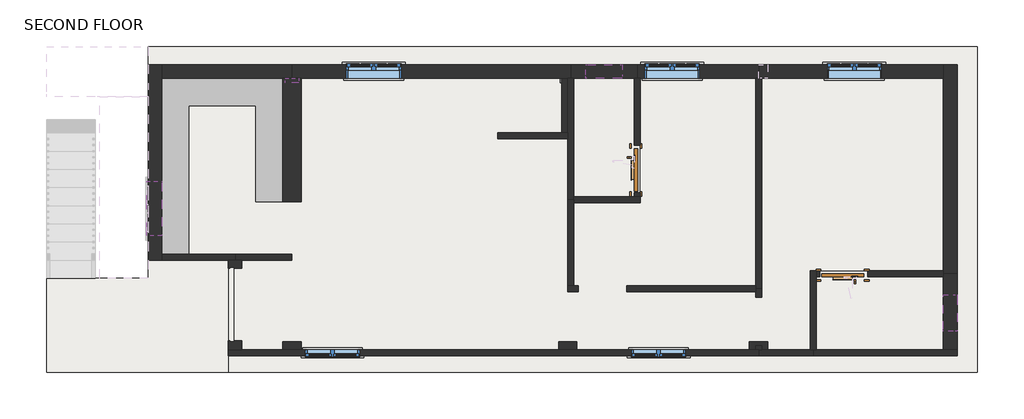
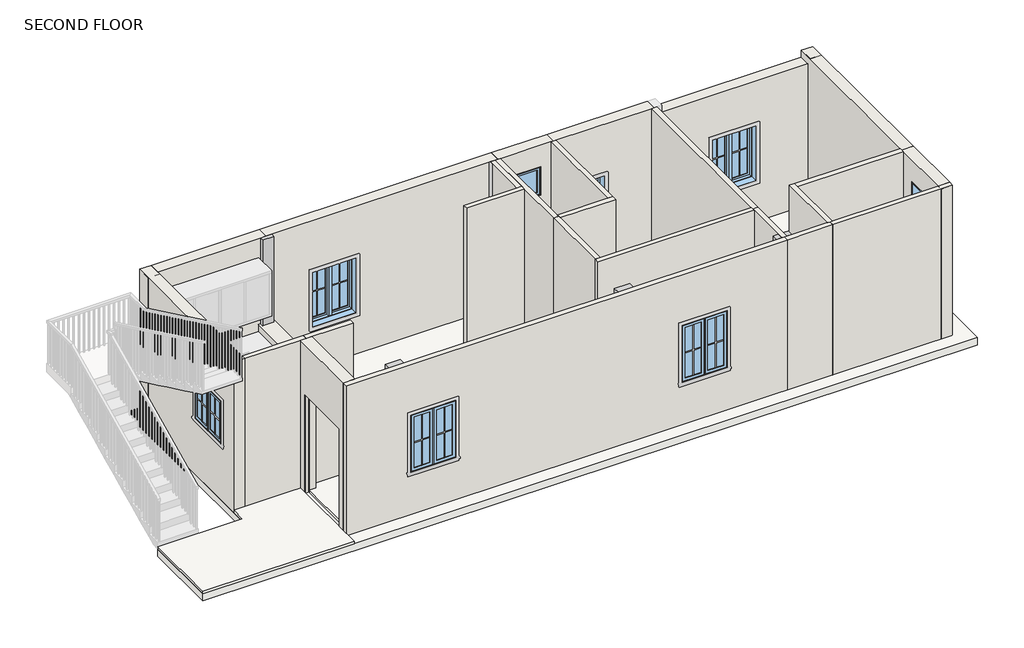
# One storey, part 1 of 3: 26 walls, 8 windows, 6 columns, 4 slabs, 2 doors.
"""IFC4 building model written with IfcOpenShell, lengths in millimetres."""

from ifc_helpers import new_model, si_unit, frame, origin, place, context, project, spatial, polyline, outline, extrude, faceted_brep, transform, mapped, element, save
from components import apartment_toilet_door_15897_d3_toilet_d7560075, apartment_toilet_door_15897_d3_toilet_03746f18, window_80340324, window_casement_double_w1_d341e8ac, window_casement_double_w1_80f1179f, window_casement_double_w1_2_90de19e9

model = new_model("IFC4")

# Units and contexts
model_context = context("Model", 3, world=origin())
ifc_project = project(units=[si_unit("LENGTHUNIT", "METRE", prefix="MILLI")], contexts=[model_context])

# Site, building, storey
site = spatial("IfcSite", under=ifc_project)
building = spatial("IfcBuilding", under=site)
storey = spatial("IfcBuildingStorey", under=building, Name="SECOND FLOOR", Elevation=6400.8)

# Columns
placement = place(None, origin())
element("IfcColumn", 1, ObjectType="Rectangular Column : 9\" X 12\"", at=placement, inside=storey, context=model_context, shape_type="SweptSolid", body=[
    extrude(outline(polyline([(-2166.0591227, 4797.7642852), (-2394.6591227, 4797.7642852), (-2394.6591227, 4873.9642852), (-2280.3591227, 4873.9642852), (-2166.0591227, 4873.9642852), (-2166.0591227, 4797.7642852)])), frame((0.0, 0.0, 7772.4), z_axis=(0.0, 0.0, 1.0), x_axis=(1.0, 0.0, 0.0)), (0.0, 0.0, 1.0), 1828.8),
])
element("IfcColumn", 2, ObjectType="Rectangular Column : 9\" X 12\"", at=placement, inside=storey, context=model_context, shape_type="Brep", body=[
    faceted_brep([(-4693.3591227, 5102.5642852, 6400.8), (-4464.7591227, 5102.5642852, 6400.8), (-4464.7591227, 4873.9642852, 6400.8), (-4464.7591227, 4797.7642852, 6400.8), (-4693.3591227, 4797.7642852, 6400.8), (-4693.3591227, 5102.5642852, 9601.2), (-4464.7591227, 5102.5642852, 9601.2), (-4464.7591227, 4873.9642852, 9601.2), (-4464.7591227, 4797.7642852, 9601.2), (-4693.3591227, 4797.7642852, 9601.2)], [[[0, 1, 2, 3, 4]], [[5, 6, 1, 0]], [[6, 7, 8, 3, 2, 1]], [[8, 9, 4, 3]], [[9, 5, 0, 4]], [[5, 9, 8, 7, 6]]]),
])
element("IfcColumn", 3, ObjectType="Rectangular Column : 9\" X 12\"", at=placement, inside=storey, context=model_context, shape_type="Brep", body=[
    faceted_brep([(5390.4408773, 454.3642852, 6400.8), (5695.2408773, 454.3642852, 6400.8), (5695.2408773, 327.3642852, 6400.8), (5593.6408773, 327.3642852, 6400.8), (5593.6408773, 390.8642852, 6400.8), (5492.0408773, 390.8642852, 6400.8), (5492.0408773, 327.3642852, 6400.8), (5390.4408773, 327.3642852, 6400.8), (5695.2408773, 454.3642852, 9601.2), (5695.2408773, 327.3642852, 9601.2), (5390.4408773, 454.3642852, 9601.2), (5390.4408773, 327.3642852, 9601.2), (5492.0408773, 454.3642852, 9601.2), (5492.0408773, 454.3642852, 8534.4), (5593.6408773, 454.3642852, 8534.4), (5593.6408773, 454.3642852, 9601.2), (5593.6408773, 327.3642852, 9601.2), (5593.6408773, 390.8642852, 8534.4), (5492.0408773, 390.8642852, 8534.4), (5492.0408773, 327.3642852, 9601.2)], [[[0, 1, 2, 3, 4, 5, 6, 7]], [[1, 8, 9, 2]], [[10, 0, 7, 11]], [[1, 0, 10, 12, 13, 14, 15, 8]], [[8, 15, 16, 9]], [[17, 4, 3, 16, 15, 14]], [[5, 18, 13, 12, 19, 6]], [[4, 17, 18, 5]], [[18, 17, 14, 13]], [[7, 6, 19, 11]], [[12, 10, 11, 19]], [[3, 2, 9, 16]]]),
])
element("IfcColumn", 4, ObjectType="Rectangular Column : 9\" X 12\"", at=placement, inside=storey, context=model_context, shape_type="SweptSolid", body=[
    extrude(outline(polyline([(2190.0408773, 454.3642852), (2494.8408773, 454.3642852), (2494.8408773, 327.3642852), (2190.0408773, 327.3642852), (2190.0408773, 454.3642852)])), frame((0.0, 0.0, 6400.8), z_axis=(0.0, 0.0, 1.0), x_axis=(1.0, 0.0, 0.0)), (0.0, 0.0, 1.0), 3200.4),
])
element("IfcColumn", 5, ObjectType="Rectangular Column : 9\" X 12\"", at=placement, inside=storey, context=model_context, shape_type="SweptSolid", body=[
    extrude(outline(polyline([(-2432.7591227, 454.3642852), (-2127.9591227, 454.3642852), (-2127.9591227, 327.3642852), (-2432.7591227, 327.3642852), (-2432.7591227, 454.3642852)])), frame((0.0, 0.0, 6400.8), z_axis=(0.0, 0.0, 1.0), x_axis=(1.0, 0.0, 0.0)), (0.0, 0.0, 1.0), 3200.4),
])
element("IfcColumn", 6, ObjectType="Rectangular Column : 9\" X 12\"", at=placement, inside=storey, context=model_context, shape_type="Brep", body=[
    faceted_brep([(-4693.3591227, 2130.7642852, 6400.8), (-4464.7591227, 2130.7642852, 6400.8), (-4464.7591227, 1927.5642852, 6400.8), (-4464.7591227, 1825.9642852, 6400.8), (-4693.3591227, 1825.9642852, 6400.8), (-4693.3591227, 2130.7642852, 9601.2), (-4464.7591227, 2130.7642852, 9601.2), (-4464.7591227, 1927.5642852, 9601.2), (-4464.7591227, 1825.9642852, 9601.2), (-4693.3591227, 1825.9642852, 9601.2)], [[[0, 1, 2, 3, 4]], [[5, 6, 1, 0]], [[6, 7, 8, 3, 2, 1]], [[8, 9, 4, 3]], [[9, 5, 0, 4]], [[5, 9, 8, 7, 6]]]),
])

# Doors
apartment_toilet_door_15897_d3_toilet_shape = apartment_toilet_door_15897_d3_toilet_d7560075(model_context)
element("IfcDoor", 7, ObjectType="Apartment_Toilet_Door_15897 : D3 TOILET", at=placement, inside=storey, context=model_context, shape_type="MappedRepresentation", body=[
    mapped(apartment_toilet_door_15897_d3_toilet_shape, transform((6952.5408773, 1597.3642852, 6400.8), x_axis=(-1.0, 0.0, 0.0), y_axis=(0.0, -1.0, 0.0), z_axis=(0.0, 0.0, 1.0))),
])
apartment_toilet_door_15897_d3_toilet_2_shape = apartment_toilet_door_15897_d3_toilet_03746f18(model_context)
element("IfcDoor", 8, ObjectType="Apartment_Toilet_Door_15897 : D3 TOILET", at=placement, inside=storey, context=model_context, shape_type="MappedRepresentation", body=[
    mapped(apartment_toilet_door_15897_d3_toilet_2_shape, transform((3510.8408773, 3337.2642852, 6400.8), x_axis=(0.0, -1.0, 0.0), y_axis=(1.0, 0.0, 0.0), z_axis=(0.0, 0.0, 1.0))),
])

# Slabs
element("IfcSlab", 9, ObjectType="6\" SLAB", at=placement, inside=storey, context=model_context, shape_type="SweptSolid", body=[
    extrude(outline(polyline([(9213.1408773, 5407.3642852), (9213.1408773, 113.4304234), (9213.1408773, -53.6357148), (-6395.1591227, -53.6357148), (-6395.1591227, 1521.1642852), (-4693.3591227, 1521.1642852), (-4693.3591227, 5407.3642852), (9213.1408773, 5407.3642852)])), frame((0.0, 0.0, 6248.4), z_axis=(0.0, 0.0, 1.0), x_axis=(1.0, 0.0, 0.0)), (0.0, 0.0, 1.0), 152.4),
])
element("IfcSlab", 10, ObjectType="FLOORING", at=placement, inside=storey, context=model_context, shape_type="SweptSolid", body=[
    extrude(outline(polyline([(-4464.7591227, 1927.5642852), (-4464.7591227, 4873.9642852), (-2432.7591227, 4873.9642852), (-2432.7591227, 2803.8642852), (-2127.9591227, 2803.8642852), (-2127.9591227, 4873.9642852), (2240.8408773, 4873.9642852), (2240.8408773, 3959.5642852), (1174.0408773, 3959.5642852), (1174.0408773, 3857.9642852), (2342.4408773, 3857.9642852), (2342.4408773, 1292.5642852), (2520.2408773, 1292.5642852), (2520.2408773, 1394.1642852), (2444.0408773, 1394.1642852), (2444.0408773, 2791.1642852), (3561.6408773, 2791.1642852), (3561.6408773, 4873.9642852), (5492.0408773, 4873.9642852), (5492.0408773, 1394.1642852), (3409.2408773, 1394.1642852), (3333.0408773, 1394.1642852), (3333.0408773, 1292.5642852), (5492.0408773, 1292.5642852), (5492.0408773, 1203.6642852), (5593.6408773, 1203.6642852), (5593.6408773, 4873.9642852), (8641.6408773, 4873.9642852), (8641.6408773, 1648.1642852), (6406.4408773, 1648.1642852), (6406.4408773, 327.3642852), (5593.6408773, 327.3642852), (5593.6408773, 390.8642852), (5492.0408773, 390.8642852), (5492.0408773, 327.3642852), (-3118.5591227, 327.3642852), (-3118.5591227, 397.6642852), (-3250.1591227, 397.6642852), (-3250.1591227, 1769.2642852), (-3118.5591227, 1769.2642852), (-3118.5591227, 1825.9642852), (-2280.3591227, 1825.9642852), (-2280.3591227, 1927.5642852), (-4464.7591227, 1927.5642852)])), frame((0.0, 0.0, 6400.8), z_axis=(0.0, 0.0, 1.0), x_axis=(1.0, 0.0, 0.0)), (0.0, 0.0, 1.0), 50.8),
])
element("IfcSlab", 11, ObjectType="FLOORING OPEN AREA", at=placement, inside=storey, context=model_context, shape_type="SweptSolid", body=[
    extrude(outline(polyline([(-3347.1591227, -53.6357148), (-6395.1591227, -53.6357148), (-6395.1591227, 1521.1642852), (-4693.3591227, 1521.1642852), (-4693.3591227, 1825.9642852), (-3347.1591227, 1825.9642852), (-3347.1591227, -53.6357148)])), frame((0.0, 0.0, 6400.8), z_axis=(0.0, 0.0, 1.0), x_axis=(1.0, 0.0, 0.0)), (0.0, 0.0, 1.0), 50.8),
])
element("IfcSlab", 12, ObjectType="FLOORING TOILET", at=placement, inside=storey, context=model_context, shape_type="SweptSolid", body=[
    extrude(outline(polyline([(7371.5408773, 1546.5642852), (8641.6408773, 1546.5642852), (8641.6408773, 327.3642852), (6508.0408773, 327.3642852), (6508.0408773, 1546.5642852), (6571.5408773, 1546.5642852), (6571.5408773, 1648.1642852), (7371.5408773, 1648.1642852), (7371.5408773, 1546.5642852)])), frame((0.0, 0.0, 6400.8), z_axis=(0.0, 0.0, 1.0), x_axis=(1.0, 0.0, 0.0)), (0.0, 0.0, 1.0), 50.8),
    extrude(outline(polyline([(3460.0408773, 4873.9642852), (3460.0408773, 3756.2642852), (3561.6408773, 3756.2642852), (3561.6408773, 2956.2642852), (3460.0408773, 2956.2642852), (3460.0408773, 2892.7642852), (2444.0408773, 2892.7642852), (2444.0408773, 4873.9642852), (3460.0408773, 4873.9642852)])), frame((0.0, 0.0, 6400.8), z_axis=(0.0, 0.0, 1.0), x_axis=(1.0, 0.0, 0.0)), (0.0, 0.0, 1.0), 50.8),
])

# Walls
element("IfcWall", 13, at=placement, inside=storey, context=model_context, shape_type="Brep", body=[
    faceted_brep([(-2432.7591227, 4873.9642852, 6400.8), (-2432.7591227, 2803.8642852, 6400.8), (-2432.7591227, 2803.8642852, 7772.4), (-2432.7591227, 4873.9642852, 7772.4), (-2127.9591227, 4873.9642852, 6400.8), (-2127.9591227, 4873.9642852, 7772.4), (-2127.9591227, 2803.8642852, 7772.4), (-2127.9591227, 2803.8642852, 6400.8), (-2280.3591227, 4873.9642852, 6400.8), (-2166.0591227, 4873.9642852, 7772.4), (-2280.3591227, 4873.9642852, 7772.4), (-2394.6591227, 4873.9642852, 7772.4)], [[[0, 1, 2, 3]], [[4, 5, 6, 7]], [[1, 0, 8, 4, 7]], [[2, 1, 7, 6]], [[3, 2, 6, 5, 9, 10, 11]], [[0, 3, 11, 10, 9, 5, 4, 8]]]),
])
element("IfcWall", 14, ObjectType="4\" WALL", at=placement, inside=storey, context=model_context, shape_type="Brep", body=[
    faceted_brep([(8870.2408773, 327.3642852, 6400.8), (8641.6408773, 327.3642852, 6400.8), (6508.0408773, 327.3642852, 6400.8), (6457.2408773, 327.3642852, 6400.8), (6457.2408773, 327.3642852, 9601.2), (6508.0408773, 327.3642852, 9601.2), (8641.6408773, 327.3642852, 9601.2), (8870.2408773, 327.3642852, 9601.2), (8870.2408773, 225.7642852, 6400.8), (8870.2408773, 225.7642852, 9601.2), (6457.2408773, 225.7642852, 9601.2), (6457.2408773, 225.7642852, 6400.8)], [[[0, 1, 2, 3, 4, 5, 6, 7]], [[8, 9, 10, 11]], [[3, 2, 1, 0, 8, 11]], [[4, 3, 11, 10]], [[7, 6, 5, 4, 10, 9]], [[0, 7, 9, 8]]]),
])
element("IfcWall", 15, ObjectType="4\" WALL", at=placement, inside=storey, context=model_context, shape_type="Brep", body=[
    faceted_brep([(-2280.3591227, 1927.5642852, 6400.8), (-3232.8591227, 1927.5642852, 6400.8), (-3232.8591227, 1927.5642852, 9601.2), (-2280.3591227, 1927.5642852, 9601.2), (-2280.3591227, 1825.9642852, 6400.8), (-2280.3591227, 1825.9642852, 9601.2), (-3118.5591227, 1825.9642852, 9601.2), (-3232.8591227, 1825.9642852, 9601.2), (-3232.8591227, 1825.9642852, 6400.8), (-3118.5591227, 1825.9642852, 6400.8)], [[[0, 1, 2, 3]], [[4, 5, 6, 7, 8, 9]], [[1, 0, 4, 9, 8]], [[2, 1, 8, 7]], [[3, 2, 7, 6, 5]], [[0, 3, 5, 4]]]),
])
element("IfcWall", 16, ObjectType="4\" WALL", at=placement, inside=storey, context=model_context, shape_type="Brep", body=[
    faceted_brep([(5593.6408773, 1343.3642852, 6400.8), (5593.6408773, 1343.3642852, 9601.2), (5593.6408773, 454.3642852, 9601.2), (5593.6408773, 327.3642852, 9601.2), (5593.6408773, 327.3642852, 6400.8), (5593.6408773, 390.8642852, 6400.8), (5593.6408773, 390.8642852, 8534.4), (5593.6408773, 454.3642852, 8534.4), (5593.6408773, 1203.6642852, 8534.4), (5593.6408773, 1203.6642852, 6400.8), (5492.0408773, 1343.3642852, 9601.2), (5492.0408773, 1343.3642852, 6400.8), (5492.0408773, 1292.5642852, 6400.8), (5492.0408773, 1203.6642852, 6400.8), (5492.0408773, 1203.6642852, 8534.4), (5492.0408773, 454.3642852, 8534.4), (5492.0408773, 390.8642852, 8534.4), (5492.0408773, 390.8642852, 6400.8), (5492.0408773, 327.3642852, 6400.8), (5492.0408773, 327.3642852, 9601.2), (5492.0408773, 454.3642852, 9601.2), (5492.0408773, 1292.5642852, 9601.2), (5542.8408773, 327.3642852, 6400.8), (5542.8408773, 327.3642852, 9601.2)], [[[0, 1, 2, 3, 4, 5, 6, 7, 8, 9]], [[10, 11, 12, 13, 14, 15, 16, 17, 18, 19, 20, 21]], [[11, 0, 9, 13, 12]], [[4, 22, 18, 17, 5]], [[1, 0, 11, 10]], [[3, 2, 1, 10, 21, 20, 19, 23]], [[4, 3, 23, 19, 18, 22]], [[16, 6, 5, 17]], [[6, 16, 15, 14, 8, 7]], [[8, 14, 13, 9]]]),
])
element("IfcWall", 17, ObjectType="4\" WALL", at=placement, inside=storey, context=model_context, shape_type="Brep", body=[
    faceted_brep([(5492.0408773, 1394.1642852, 6400.8), (3333.0408773, 1394.1642852, 6400.8), (3333.0408773, 1394.1642852, 8534.4), (2520.2408773, 1394.1642852, 8534.4), (2520.2408773, 1394.1642852, 6400.8), (2444.0408773, 1394.1642852, 6400.8), (2342.4408773, 1394.1642852, 6400.8), (2342.4408773, 1394.1642852, 9601.2), (2444.0408773, 1394.1642852, 9601.2), (5492.0408773, 1394.1642852, 9601.2), (3333.0408773, 1292.5642852, 8534.4), (3333.0408773, 1292.5642852, 6400.8), (5492.0408773, 1292.5642852, 6400.8), (5492.0408773, 1292.5642852, 9601.2), (2342.4408773, 1292.5642852, 9601.2), (2342.4408773, 1292.5642852, 6400.8), (2520.2408773, 1292.5642852, 6400.8), (2520.2408773, 1292.5642852, 8534.4), (5492.0408773, 1343.3642852, 6400.8), (5492.0408773, 1343.3642852, 9601.2)], [[[0, 1, 2, 3, 4, 5, 6, 7, 8, 9]], [[10, 11, 12, 13, 14, 15, 16, 17]], [[16, 15, 6, 5, 4]], [[12, 11, 1, 0, 18]], [[9, 8, 7, 14, 13, 19]], [[0, 9, 19, 13, 12, 18]], [[7, 6, 15, 14]], [[2, 1, 11, 10]], [[3, 2, 10, 17]], [[4, 3, 17, 16]]]),
])
element("IfcWall", 18, ObjectType="4\" WALL", at=placement, inside=storey, context=model_context, shape_type="Brep", body=[
    faceted_brep([(2444.0408773, 1394.1642852, 6400.8), (2444.0408773, 2791.1642852, 6400.8), (2444.0408773, 2841.9642852, 6400.8), (2444.0408773, 2841.9642852, 9601.2), (2444.0408773, 2791.1642852, 9601.2), (2444.0408773, 1394.1642852, 9601.2), (2342.4408773, 1394.1642852, 6400.8), (2342.4408773, 1394.1642852, 9601.2), (2342.4408773, 2841.9642852, 9601.2), (2342.4408773, 2841.9642852, 6400.8)], [[[0, 1, 2, 3, 4, 5]], [[6, 7, 8, 9]], [[2, 1, 0, 6, 9]], [[3, 2, 9, 8]], [[5, 4, 3, 8, 7]], [[0, 5, 7, 6]]]),
])
element("IfcWall", 19, ObjectType="4\" WALL", at=placement, inside=storey, context=model_context, shape_type="Brep", body=[
    faceted_brep([(2342.4408773, 3959.5642852, 6400.8), (2240.8408773, 3959.5642852, 6400.8), (1174.0408773, 3959.5642852, 6400.8), (1174.0408773, 3959.5642852, 9601.2), (2240.8408773, 3959.5642852, 9601.2), (2342.4408773, 3959.5642852, 9601.2), (2342.4408773, 3857.9642852, 6400.8), (2342.4408773, 3857.9642852, 9601.2), (1174.0408773, 3857.9642852, 9601.2), (1174.0408773, 3857.9642852, 6400.8)], [[[0, 1, 2, 3, 4, 5]], [[6, 7, 8, 9]], [[2, 1, 0, 6, 9]], [[3, 2, 9, 8]], [[5, 4, 3, 8, 7]], [[0, 5, 7, 6]]]),
])
element("IfcWall", 20, ObjectType="4\" WALL", at=placement, inside=storey, context=model_context, shape_type="Brep", body=[
    faceted_brep([(6508.0408773, 327.3642852, 6400.8), (6508.0408773, 1546.5642852, 6400.8), (6508.0408773, 1648.1642852, 6400.8), (6508.0408773, 1648.1642852, 9601.2), (6508.0408773, 1546.5642852, 9601.2), (6508.0408773, 327.3642852, 9601.2), (6406.4408773, 327.3642852, 6400.8), (6406.4408773, 327.3642852, 9601.2), (6406.4408773, 1648.1642852, 9601.2), (6406.4408773, 1648.1642852, 6400.8), (6457.2408773, 327.3642852, 6400.8), (6457.2408773, 327.3642852, 9601.2)], [[[0, 1, 2, 3, 4, 5]], [[6, 7, 8, 9]], [[2, 1, 0, 10, 6, 9]], [[5, 4, 3, 8, 7, 11]], [[0, 5, 11, 7, 6, 10]], [[3, 2, 9, 8]]]),
])
element("IfcWall", 21, ObjectType="4\" WALL", at=placement, inside=storey, context=model_context, shape_type="Brep", body=[
    faceted_brep([(6508.0408773, 1546.5642852, 6400.8), (6571.5408773, 1546.5642852, 6400.8), (6571.5408773, 1546.5642852, 8534.4), (7371.5408773, 1546.5642852, 8534.4), (7371.5408773, 1546.5642852, 6400.8), (8641.6408773, 1546.5642852, 6400.8), (8641.6408773, 1546.5642852, 9601.2), (6508.0408773, 1546.5642852, 9601.2), (6571.5408773, 1648.1642852, 8534.4), (6571.5408773, 1648.1642852, 6400.8), (6508.0408773, 1648.1642852, 6400.8), (6508.0408773, 1648.1642852, 9601.2), (8641.6408773, 1648.1642852, 9601.2), (8641.6408773, 1648.1642852, 6400.8), (7371.5408773, 1648.1642852, 6400.8), (7371.5408773, 1648.1642852, 8534.4), (8641.6408773, 1597.3642852, 6400.8), (8641.6408773, 1597.3642852, 9601.2)], [[[0, 1, 2, 3, 4, 5, 6, 7]], [[8, 9, 10, 11, 12, 13, 14, 15]], [[14, 13, 16, 5, 4]], [[10, 9, 1, 0]], [[7, 6, 17, 12, 11]], [[0, 7, 11, 10]], [[6, 5, 16, 13, 12, 17]], [[2, 1, 9, 8]], [[3, 2, 8, 15]], [[4, 3, 15, 14]]]),
])
element("IfcWall", 22, ObjectType="4\" WALL", at=placement, inside=storey, context=model_context, shape_type="Brep", body=[
    faceted_brep([(2444.0408773, 2791.1642852, 6400.8), (3561.6408773, 2791.1642852, 6400.8), (3561.6408773, 2791.1642852, 9601.2), (2444.0408773, 2791.1642852, 9601.2), (2444.0408773, 2892.7642852, 6400.8), (2444.0408773, 2892.7642852, 9601.2), (3460.0408773, 2892.7642852, 9601.2), (3561.6408773, 2892.7642852, 9601.2), (3561.6408773, 2892.7642852, 6400.8), (3460.0408773, 2892.7642852, 6400.8), (2444.0408773, 2841.9642852, 6400.8), (2444.0408773, 2841.9642852, 9601.2)], [[[0, 1, 2, 3]], [[4, 5, 6, 7, 8, 9]], [[1, 0, 10, 4, 9, 8]], [[3, 2, 7, 6, 5, 11]], [[0, 3, 11, 5, 4, 10]], [[2, 1, 8, 7]]]),
])
element("IfcWall", 23, ObjectType="4\" WALL", at=placement, inside=storey, context=model_context, shape_type="Brep", body=[
    faceted_brep([(3561.6408773, 2892.7642852, 6400.8), (3561.6408773, 2956.2642852, 6400.8), (3561.6408773, 2956.2642852, 8534.4), (3561.6408773, 3756.2642852, 8534.4), (3561.6408773, 3756.2642852, 6400.8), (3561.6408773, 4873.9642852, 6400.8), (3561.6408773, 4873.9642852, 9601.2), (3561.6408773, 2892.7642852, 9601.2), (3460.0408773, 2956.2642852, 8534.4), (3460.0408773, 2956.2642852, 6400.8), (3460.0408773, 2892.7642852, 6400.8), (3460.0408773, 2892.7642852, 9601.2), (3460.0408773, 4873.9642852, 9601.2), (3460.0408773, 4873.9642852, 6400.8), (3460.0408773, 3756.2642852, 6400.8), (3460.0408773, 3756.2642852, 8534.4), (3510.8408773, 4873.9642852, 6400.8), (3510.8408773, 4873.9642852, 9601.2)], [[[0, 1, 2, 3, 4, 5, 6, 7]], [[8, 9, 10, 11, 12, 13, 14, 15]], [[14, 13, 16, 5, 4]], [[10, 9, 1, 0]], [[7, 6, 17, 12, 11]], [[0, 7, 11, 10]], [[6, 5, 16, 13, 12, 17]], [[2, 1, 9, 8]], [[3, 2, 8, 15]], [[4, 3, 15, 14]]]),
])
element("IfcWall", 24, ObjectType="4\" WALL", at=placement, inside=storey, context=model_context, shape_type="Brep", body=[
    faceted_brep([(2342.4408773, 3959.5642852, 6400.8), (2342.4408773, 4873.9642852, 6400.8), (2342.4408773, 4873.9642852, 9601.2), (2342.4408773, 3959.5642852, 9601.2), (2240.8408773, 3959.5642852, 6400.8), (2240.8408773, 3959.5642852, 9601.2), (2240.8408773, 4797.7642852, 9601.2), (2240.8408773, 4873.9642852, 9601.2), (2240.8408773, 4873.9642852, 6400.8), (2240.8408773, 4797.7642852, 6400.8)], [[[0, 1, 2, 3]], [[4, 5, 6, 7, 8, 9]], [[1, 0, 4, 9, 8]], [[3, 2, 7, 6, 5]], [[2, 1, 8, 7]], [[0, 3, 5, 4]]]),
])
element("IfcWall", 25, ObjectType="4\" WALL", at=placement, inside=storey, context=model_context, shape_type="Brep", body=[
    faceted_brep([(2444.0408773, 2841.9642852, 6400.8), (2444.0408773, 2892.7642852, 6400.8), (2444.0408773, 4873.9642852, 6400.8), (2444.0408773, 4873.9642852, 9601.2), (2444.0408773, 2892.7642852, 9601.2), (2444.0408773, 2841.9642852, 9601.2), (2342.4408773, 2841.9642852, 6400.8), (2342.4408773, 2841.9642852, 9601.2), (2342.4408773, 3857.9642852, 9601.2), (2342.4408773, 3959.5642852, 9601.2), (2342.4408773, 4873.9642852, 9601.2), (2342.4408773, 4873.9642852, 6400.8), (2342.4408773, 3959.5642852, 6400.8), (2342.4408773, 3857.9642852, 6400.8), (2393.2408773, 4873.9642852, 6400.8), (2393.2408773, 4873.9642852, 9601.2)], [[[0, 1, 2, 3, 4, 5]], [[6, 7, 8, 9, 10, 11, 12, 13]], [[2, 1, 0, 6, 13, 12, 11, 14]], [[5, 4, 3, 15, 10, 9, 8, 7]], [[0, 5, 7, 6]], [[3, 2, 14, 11, 10, 15]]]),
])
element("IfcWall", 26, ObjectType="4\" WALL", at=placement, inside=storey, context=model_context, shape_type="Brep", body=[
    faceted_brep([(-3232.8591227, 1927.5642852, 6400.8), (-4464.7591227, 1927.5642852, 6400.8), (-4464.7591227, 1927.5642852, 9601.2), (-3232.8591227, 1927.5642852, 9601.2), (-3232.8591227, 1825.9642852, 6400.8), (-3232.8591227, 1825.9642852, 9601.2), (-3347.1591227, 1825.9642852, 9601.2), (-4464.7591227, 1825.9642852, 9601.2), (-4464.7591227, 1825.9642852, 6400.8), (-3347.1591227, 1825.9642852, 6400.8)], [[[0, 1, 2, 3]], [[4, 5, 6, 7, 8, 9]], [[1, 0, 4, 9, 8]], [[3, 2, 7, 6, 5]], [[0, 3, 5, 4]], [[2, 1, 8, 7]]]),
])
element("IfcWall", 27, ObjectType="4\" WALL", at=placement, inside=storey, context=model_context, shape_type="Brep", body=[
    faceted_brep([(5593.6408773, 1343.3642852, 6400.8), (5593.6408773, 4873.9642852, 6400.8), (5593.6408773, 4873.9642852, 9601.2), (5593.6408773, 1343.3642852, 9601.2), (5492.0408773, 1343.3642852, 6400.8), (5492.0408773, 1343.3642852, 9601.2), (5492.0408773, 1394.1642852, 9601.2), (5492.0408773, 4873.9642852, 9601.2), (5492.0408773, 4873.9642852, 6400.8), (5492.0408773, 1394.1642852, 6400.8), (5542.8408773, 4873.9642852, 6400.8), (5542.8408773, 4873.9642852, 9601.2)], [[[0, 1, 2, 3]], [[4, 5, 6, 7, 8, 9]], [[1, 0, 4, 9, 8, 10]], [[3, 2, 11, 7, 6, 5]], [[0, 3, 5, 4]], [[2, 1, 10, 8, 7, 11]]]),
])
element("IfcWall", 28, ObjectType="4\" WALL", at=placement, inside=storey, context=model_context, shape_type="Brep", body=[
    faceted_brep([(5542.8408773, 327.3642852, 6400.8), (5492.0408773, 327.3642852, 6400.8), (5390.4408773, 327.3642852, 6400.8), (2494.8408773, 327.3642852, 6400.8), (2190.0408773, 327.3642852, 6400.8), (-2127.9591227, 327.3642852, 6400.8), (-2432.7591227, 327.3642852, 6400.8), (-3118.5591227, 327.3642852, 6400.8), (-3347.1591227, 327.3642852, 6400.8), (-3347.1591227, 327.3642852, 9601.2), (-3118.5591227, 327.3642852, 9601.2), (-2432.7591227, 327.3642852, 9601.2), (-2127.9591227, 327.3642852, 9601.2), (2190.0408773, 327.3642852, 9601.2), (2494.8408773, 327.3642852, 9601.2), (5390.4408773, 327.3642852, 9601.2), (5492.0408773, 327.3642852, 9601.2), (5542.8408773, 327.3642852, 9601.2), (3409.2408773, 327.3642852, 8534.4), (3409.2408773, 327.3642852, 7315.2), (4323.6408773, 327.3642852, 7315.2), (4323.6408773, 327.3642852, 8534.4), (-2058.1091227, 327.3642852, 8534.4), (-2058.1091227, 327.3642852, 7315.2), (-1143.7091227, 327.3642852, 7315.2), (-1143.7091227, 327.3642852, 8534.4), (-3347.1591227, 225.7642852, 6400.8), (5542.8408773, 225.7642852, 6400.8), (5542.8408773, 225.7642852, 9601.2), (-3347.1591227, 225.7642852, 9601.2), (3409.2408773, 225.7642852, 8534.4), (4323.6408773, 225.7642852, 8534.4), (4323.6408773, 225.7642852, 7315.2), (3409.2408773, 225.7642852, 7315.2), (-2058.1091227, 225.7642852, 7315.2), (-2058.1091227, 225.7642852, 8534.4), (-1143.7091227, 225.7642852, 8534.4), (-1143.7091227, 225.7642852, 7315.2)], [[[0, 1, 2, 3, 4, 5, 6, 7, 8, 9, 10, 11, 12, 13, 14, 15, 16, 17], [18, 19, 20, 21], [22, 23, 24, 25]], [[26, 27, 28, 29], [30, 31, 32, 33], [34, 35, 36, 37]], [[8, 7, 6, 5, 4, 3, 2, 1, 0, 27, 26]], [[17, 16, 15, 14, 13, 12, 11, 10, 9, 29, 28]], [[0, 17, 28, 27]], [[9, 8, 26, 29]], [[18, 21, 31, 30]], [[21, 20, 32, 31]], [[20, 19, 33, 32]], [[19, 18, 30, 33]], [[22, 35, 34, 23]], [[23, 34, 37, 24]], [[24, 37, 36, 25]], [[35, 22, 25, 36]]]),
])
element("IfcWall", 29, ObjectType="4\" WALL", at=placement, inside=storey, context=model_context, shape_type="Brep", body=[
    faceted_brep([(6457.2408773, 327.3642852, 6400.8), (6406.4408773, 327.3642852, 6400.8), (5695.2408773, 327.3642852, 6400.8), (5593.6408773, 327.3642852, 6400.8), (5542.8408773, 327.3642852, 6400.8), (5542.8408773, 327.3642852, 9601.2), (5593.6408773, 327.3642852, 9601.2), (5695.2408773, 327.3642852, 9601.2), (6406.4408773, 327.3642852, 9601.2), (6457.2408773, 327.3642852, 9601.2), (6457.2408773, 225.7642852, 6400.8), (6457.2408773, 225.7642852, 9601.2), (5542.8408773, 225.7642852, 9601.2), (5542.8408773, 225.7642852, 6400.8)], [[[0, 1, 2, 3, 4, 5, 6, 7, 8, 9]], [[10, 11, 12, 13]], [[4, 3, 2, 1, 0, 10, 13]], [[5, 4, 13, 12]], [[9, 8, 7, 6, 5, 12, 11]], [[0, 9, 11, 10]]]),
])
element("IfcWall", 30, ObjectType="9\" WALL", at=placement, inside=storey, context=model_context, shape_type="Brep", body=[
    faceted_brep([(8641.6408773, 5102.5642852, 6400.8), (5542.8408773, 5102.5642852, 6400.8), (5542.8408773, 5102.5642852, 9448.8), (5695.2408773, 5102.5642852, 9448.8), (8641.6408773, 5102.5642852, 9448.8), (7606.5908773, 5102.5642852, 8534.4), (6692.1908773, 5102.5642852, 8534.4), (6692.1908773, 5102.5642852, 7315.2), (7606.5908773, 5102.5642852, 7315.2), (8641.6408773, 4873.9642852, 6400.8), (8641.6408773, 4873.9642852, 9448.8), (5695.2408773, 4873.9642852, 9448.8), (5542.8408773, 4873.9642852, 9448.8), (5542.8408773, 4873.9642852, 6400.8), (5593.6408773, 4873.9642852, 6400.8), (7606.5908773, 4873.9642852, 8534.4), (7606.5908773, 4873.9642852, 7315.2), (6692.1908773, 4873.9642852, 7315.2), (6692.1908773, 4873.9642852, 8534.4)], [[[0, 1, 2, 3, 4], [5, 6, 7, 8]], [[9, 10, 11, 12, 13, 14], [15, 16, 17, 18]], [[1, 0, 9, 14, 13]], [[2, 1, 13, 12]], [[0, 4, 10, 9]], [[16, 15, 5, 8]], [[17, 16, 8, 7]], [[18, 17, 7, 6]], [[15, 18, 6, 5]], [[4, 3, 2, 12, 11, 10]]]),
])
element("IfcWall", 31, ObjectType="9\" WALL", at=placement, inside=storey, context=model_context, shape_type="Brep", body=[
    faceted_brep([(8870.2408773, 327.3642852, 6400.8), (8870.2408773, 1597.3642852, 6400.8), (8870.2408773, 1597.3642852, 9601.2), (8870.2408773, 327.3642852, 9601.2), (8870.2408773, 632.1642852, 9144.0), (8870.2408773, 1241.7642852, 9144.0), (8870.2408773, 1241.7642852, 8534.4), (8870.2408773, 632.1642852, 8534.4), (8641.6408773, 327.3642852, 6400.8), (8641.6408773, 327.3642852, 9601.2), (8641.6408773, 1546.5642852, 9601.2), (8641.6408773, 1597.3642852, 9601.2), (8641.6408773, 1597.3642852, 6400.8), (8641.6408773, 1546.5642852, 6400.8), (8641.6408773, 632.1642852, 9144.0), (8641.6408773, 632.1642852, 8534.4), (8641.6408773, 1241.7642852, 8534.4), (8641.6408773, 1241.7642852, 9144.0)], [[[0, 1, 2, 3], [4, 5, 6, 7]], [[8, 9, 10, 11, 12, 13], [14, 15, 16, 17]], [[1, 0, 8, 13, 12]], [[2, 1, 12, 11]], [[3, 2, 11, 10, 9]], [[0, 3, 9, 8]], [[15, 14, 4, 7]], [[16, 15, 7, 6]], [[17, 16, 6, 5]], [[14, 17, 5, 4]]]),
])
element("IfcWall", 32, ObjectType="9\" WALL", at=placement, inside=storey, context=model_context, shape_type="Brep", body=[
    faceted_brep([(-4464.7591227, 1825.9642852, 6400.8), (-4464.7591227, 1927.5642852, 6400.8), (-4464.7591227, 4873.9642852, 6400.8), (-4464.7591227, 5102.5642852, 6400.8), (-4464.7591227, 5102.5642852, 9601.2), (-4464.7591227, 4873.9642852, 9601.2), (-4464.7591227, 1927.5642852, 9601.2), (-4464.7591227, 1825.9642852, 9601.2), (-4464.7591227, 3146.7642852, 8534.4), (-4464.7591227, 3146.7642852, 7620.0), (-4464.7591227, 2232.3642852, 7620.0), (-4464.7591227, 2232.3642852, 8534.4), (-4693.3591227, 1825.9642852, 6400.8), (-4693.3591227, 1825.9642852, 9601.2), (-4693.3591227, 5102.5642852, 9601.2), (-4693.3591227, 5102.5642852, 6400.8), (-4693.3591227, 3146.7642852, 8534.4), (-4693.3591227, 2232.3642852, 8534.4), (-4693.3591227, 2232.3642852, 7620.0), (-4693.3591227, 3146.7642852, 7620.0)], [[[0, 1, 2, 3, 4, 5, 6, 7], [8, 9, 10, 11]], [[12, 13, 14, 15], [16, 17, 18, 19]], [[3, 2, 1, 0, 12, 15]], [[7, 6, 5, 4, 14, 13]], [[4, 3, 15, 14]], [[0, 7, 13, 12]], [[9, 8, 16, 19]], [[10, 9, 19, 18]], [[11, 10, 18, 17]], [[8, 11, 17, 16]]]),
])
element("IfcWall", 33, ObjectType="9\" WALL", at=placement, inside=storey, context=model_context, shape_type="Brep", body=[
    faceted_brep([(-3118.5591227, 1825.9642852, 9601.2), (-3118.5591227, 327.3642852, 9601.2), (-3118.5591227, 327.3642852, 6400.8), (-3118.5591227, 473.8642852, 6400.8), (-3118.5591227, 473.8642852, 8534.4), (-3118.5591227, 1693.0642852, 8534.4), (-3118.5591227, 1693.0642852, 6400.8), (-3118.5591227, 1825.9642852, 6400.8), (-3347.1591227, 327.3642852, 9601.2), (-3347.1591227, 1825.9642852, 9601.2), (-3347.1591227, 1825.9642852, 6400.8), (-3347.1591227, 1693.0642852, 6400.8), (-3347.1591227, 1693.0642852, 8534.4), (-3347.1591227, 473.8642852, 8534.4), (-3347.1591227, 473.8642852, 6400.8), (-3347.1591227, 327.3642852, 6400.8), (-3327.1591227, 473.8642852, 6400.8), (-3327.1591227, 458.8642852, 6400.8), (-3250.1591227, 458.8642852, 6400.8), (-3250.1591227, 473.8642852, 6400.8), (-3232.8591227, 1825.9642852, 6400.8), (-3250.1591227, 1693.0642852, 6400.8), (-3250.1591227, 1708.0642852, 6400.8), (-3327.1591227, 1708.0642852, 6400.8), (-3327.1591227, 1693.0642852, 6400.8), (-3232.8591227, 1825.9642852, 9601.2), (-3327.1591227, 1693.0642852, 8534.4), (-3327.1591227, 473.8642852, 8534.4), (-3327.1591227, 1708.0642852, 8549.4), (-3327.1591227, 458.8642852, 8549.4), (-3250.1591227, 1708.0642852, 8549.4), (-3250.1591227, 1693.0642852, 8534.4), (-3250.1591227, 473.8642852, 8534.4), (-3250.1591227, 458.8642852, 8549.4)], [[[0, 1, 2, 3, 4, 5, 6, 7]], [[8, 9, 10, 11, 12, 13, 14, 15]], [[2, 15, 14, 16, 17, 18, 19, 3]], [[10, 20, 7, 6, 21, 22, 23, 24, 11]], [[1, 0, 25, 9, 8]], [[2, 1, 8, 15]], [[24, 26, 12, 11]], [[27, 16, 14, 13]], [[26, 27, 13, 12]], [[26, 24, 23, 28, 29, 17, 16, 27]], [[28, 23, 22, 30]], [[30, 22, 21, 31, 32, 19, 18, 33]], [[29, 28, 30, 33]], [[17, 29, 33, 18]], [[31, 21, 6, 5]], [[19, 32, 4, 3]], [[32, 31, 5, 4]], [[0, 7, 20, 10, 9, 25]]]),
])
element("IfcWall", 34, ObjectType="9\" WALL", at=placement, inside=storey, context=model_context, shape_type="Brep", body=[
    faceted_brep([(-2280.3591227, 5102.5642852, 9601.2), (-2280.3591227, 5102.5642852, 6400.8), (-4464.7591227, 5102.5642852, 6400.8), (-4464.7591227, 5102.5642852, 9601.2), (-2280.3591227, 4873.9642852, 6400.8), (-2280.3591227, 4873.9642852, 9601.2), (-2394.6591227, 4873.9642852, 9601.2), (-4464.7591227, 4873.9642852, 9601.2), (-4464.7591227, 4873.9642852, 6400.8), (-2432.7591227, 4873.9642852, 6400.8)], [[[0, 1, 2, 3]], [[4, 5, 6, 7, 8, 9]], [[2, 1, 4, 9, 8]], [[0, 3, 7, 6, 5]], [[3, 2, 8, 7]], [[0, 5, 4, 1]]]),
])
element("IfcWall", 35, ObjectType="9\" WALL", at=placement, inside=storey, context=model_context, shape_type="Brep", body=[
    faceted_brep([(2393.2408773, 5102.5642852, 6400.8), (-2280.3591227, 5102.5642852, 6400.8), (-2280.3591227, 5102.5642852, 9601.2), (2393.2408773, 5102.5642852, 9601.2), (-451.5591227, 5102.5642852, 8534.4), (-1365.9591227, 5102.5642852, 8534.4), (-1365.9591227, 5102.5642852, 7315.2), (-451.5591227, 5102.5642852, 7315.2), (2393.2408773, 4873.9642852, 6400.8), (2393.2408773, 4873.9642852, 9601.2), (2342.4408773, 4873.9642852, 9601.2), (2240.8408773, 4873.9642852, 9601.2), (2215.4408773, 4873.9642852, 9601.2), (-2166.0591227, 4873.9642852, 9601.2), (-2280.3591227, 4873.9642852, 9601.2), (-2280.3591227, 4873.9642852, 6400.8), (-2127.9591227, 4873.9642852, 6400.8), (2215.4408773, 4873.9642852, 6400.8), (2240.8408773, 4873.9642852, 6400.8), (2342.4408773, 4873.9642852, 6400.8), (-451.5591227, 4873.9642852, 8534.4), (-451.5591227, 4873.9642852, 7315.2), (-1365.9591227, 4873.9642852, 7315.2), (-1365.9591227, 4873.9642852, 8534.4)], [[[0, 1, 2, 3], [4, 5, 6, 7]], [[8, 9, 10, 11, 12, 13, 14, 15, 16, 17, 18, 19], [20, 21, 22, 23]], [[1, 0, 8, 19, 18, 17, 16, 15]], [[3, 2, 14, 13, 12, 11, 10, 9]], [[0, 3, 9, 8]], [[1, 15, 14, 2]], [[20, 23, 5, 4]], [[23, 22, 6, 5]], [[22, 21, 7, 6]], [[21, 20, 4, 7]]]),
])
element("IfcWall", 36, ObjectType="9\" WALL", at=placement, inside=storey, context=model_context, shape_type="Brep", body=[
    faceted_brep([(5542.8408773, 5102.5642852, 6400.8), (3510.8408773, 5102.5642852, 6400.8), (3510.8408773, 5102.5642852, 9601.2), (5542.8408773, 5102.5642852, 9601.2), (5542.8408773, 5102.5642852, 9448.8), (4552.2408773, 5102.5642852, 8534.4), (3637.8408773, 5102.5642852, 8534.4), (3637.8408773, 5102.5642852, 7315.2), (4552.2408773, 5102.5642852, 7315.2), (5542.8408773, 4873.9642852, 6400.8), (5542.8408773, 4873.9642852, 9448.8), (5542.8408773, 4873.9642852, 9601.2), (5492.0408773, 4873.9642852, 9601.2), (3561.6408773, 4873.9642852, 9601.2), (3510.8408773, 4873.9642852, 9601.2), (3510.8408773, 4873.9642852, 6400.8), (3561.6408773, 4873.9642852, 6400.8), (5492.0408773, 4873.9642852, 6400.8), (4552.2408773, 4873.9642852, 8534.4), (4552.2408773, 4873.9642852, 7315.2), (3637.8408773, 4873.9642852, 7315.2), (3637.8408773, 4873.9642852, 8534.4)], [[[0, 1, 2, 3, 4], [5, 6, 7, 8]], [[9, 10, 11, 12, 13, 14, 15, 16, 17], [18, 19, 20, 21]], [[1, 0, 9, 17, 16, 15]], [[2, 1, 15, 14]], [[3, 2, 14, 13, 12, 11]], [[0, 4, 3, 11, 10, 9]], [[18, 21, 6, 5]], [[21, 20, 7, 6]], [[20, 19, 8, 7]], [[19, 18, 5, 8]]]),
])
element("IfcWall", 37, ObjectType="9\" WALL", at=placement, inside=storey, context=model_context, shape_type="Brep", body=[
    faceted_brep([(8870.2408773, 1597.3642852, 6400.8), (8870.2408773, 5102.5642852, 6400.8), (8870.2408773, 5102.5642852, 9601.2), (8870.2408773, 1597.3642852, 9601.2), (8641.6408773, 1597.3642852, 6400.8), (8641.6408773, 1597.3642852, 9601.2), (8641.6408773, 1648.1642852, 9601.2), (8641.6408773, 5102.5642852, 9601.2), (8641.6408773, 5102.5642852, 9448.8), (8641.6408773, 5102.5642852, 6400.8), (8641.6408773, 4873.9642852, 6400.8), (8641.6408773, 1648.1642852, 6400.8)], [[[0, 1, 2, 3]], [[4, 5, 6, 7, 8, 9, 10, 11]], [[1, 0, 4, 11, 10, 9]], [[3, 2, 7, 6, 5]], [[0, 3, 5, 4]], [[2, 1, 9, 8, 7]]]),
])
element("IfcWall", 38, ObjectType="9\" WALL", at=placement, inside=storey, context=model_context, shape_type="Brep", body=[
    faceted_brep([(3510.8408773, 5102.5642852, 6400.8), (2393.2408773, 5102.5642852, 6400.8), (2393.2408773, 5102.5642852, 9601.2), (3510.8408773, 5102.5642852, 9601.2), (2647.2408773, 5102.5642852, 9144.0), (2647.2408773, 5102.5642852, 8534.4), (3256.8408773, 5102.5642852, 8534.4), (3256.8408773, 5102.5642852, 9144.0), (3510.8408773, 4873.9642852, 6400.8), (3510.8408773, 4873.9642852, 9601.2), (3460.0408773, 4873.9642852, 9601.2), (2444.0408773, 4873.9642852, 9601.2), (2393.2408773, 4873.9642852, 9601.2), (2393.2408773, 4873.9642852, 6400.8), (2444.0408773, 4873.9642852, 6400.8), (3460.0408773, 4873.9642852, 6400.8), (2647.2408773, 4873.9642852, 9144.0), (3256.8408773, 4873.9642852, 9144.0), (3256.8408773, 4873.9642852, 8534.4), (2647.2408773, 4873.9642852, 8534.4)], [[[0, 1, 2, 3], [4, 5, 6, 7]], [[8, 9, 10, 11, 12, 13, 14, 15], [16, 17, 18, 19]], [[1, 0, 8, 15, 14, 13]], [[2, 1, 13, 12]], [[3, 2, 12, 11, 10, 9]], [[0, 3, 9, 8]], [[4, 7, 17, 16]], [[7, 6, 18, 17]], [[6, 5, 19, 18]], [[5, 4, 16, 19]]]),
])

# Windows
window_shape = window_80340324(model_context)
element("IfcWindow", 39, ObjectType="Fixed : 24\" x 24\"", at=placement, inside=storey, context=model_context, shape_type="MappedRepresentation", body=[
    mapped(window_shape, transform((2913.9408773, 4988.2642852, 7620.0), x_axis=(-1.0, 0.0, 0.0), y_axis=(0.0, -1.0, 0.0), z_axis=(0.0, 0.0, 1.0))),
])
element("IfcWindow", 40, ObjectType="Fixed : 24\" x 24\"", at=placement, inside=storey, context=model_context, shape_type="MappedRepresentation", body=[
    mapped(window_shape, transform((8755.9408773, 898.8642852, 7620.0), x_axis=(0.0, -1.0, 0.0), y_axis=(1.0, 0.0, 0.0), z_axis=(0.0, 0.0, 1.0))),
])
window_casement_double_w1_shape = window_casement_double_w1_d341e8ac(model_context)
element("IfcWindow", 41, ObjectType="Window-Casement-Double : w1", at=placement, inside=storey, context=model_context, shape_type="MappedRepresentation", body=[
    mapped(window_casement_double_w1_shape, transform((-908.7591227, 4988.2642852, 6400.8), x_axis=(1.0, 0.0, 0.0), y_axis=(0.0, 1.0, 0.0), z_axis=(0.0, 0.0, 1.0))),
])
element("IfcWindow", 42, ObjectType="Window-Casement-Double : w1", at=placement, inside=storey, context=model_context, shape_type="MappedRepresentation", body=[
    mapped(window_casement_double_w1_shape, transform((4095.0408773, 4988.2642852, 6400.8), x_axis=(1.0, 0.0, 0.0), y_axis=(0.0, 1.0, 0.0), z_axis=(0.0, 0.0, 1.0))),
])
element("IfcWindow", 43, ObjectType="Window-Casement-Double : w1", at=placement, inside=storey, context=model_context, shape_type="MappedRepresentation", body=[
    mapped(window_casement_double_w1_shape, transform((7149.3908773, 4988.2642852, 6400.8), x_axis=(1.0, 0.0, 0.0), y_axis=(0.0, 1.0, 0.0), z_axis=(0.0, 0.0, 1.0))),
])
window_casement_double_w1_2_shape = window_casement_double_w1_80f1179f(model_context)
element("IfcWindow", 44, ObjectType="Window-Casement-Double : w1", at=placement, inside=storey, context=model_context, shape_type="MappedRepresentation", body=[
    mapped(window_casement_double_w1_2_shape, transform((3866.4408773, 276.5642852, 6400.8), x_axis=(-1.0, 0.0, 0.0), y_axis=(0.0, -1.0, 0.0), z_axis=(0.0, 0.0, 1.0))),
])
element("IfcWindow", 45, ObjectType="Window-Casement-Double : w1", at=placement, inside=storey, context=model_context, shape_type="MappedRepresentation", body=[
    mapped(window_casement_double_w1_2_shape, transform((-1600.9091227, 276.5642852, 6400.8), x_axis=(-1.0, 0.0, 0.0), y_axis=(0.0, -1.0, 0.0), z_axis=(0.0, 0.0, 1.0))),
])
window_casement_double_w1_2_2_shape = window_casement_double_w1_2_90de19e9(model_context)
element("IfcWindow", 46, ObjectType="Window-Casement-Double : w1 2", at=placement, inside=storey, context=model_context, shape_type="MappedRepresentation", body=[
    mapped(window_casement_double_w1_2_2_shape, transform((-4579.0591227, 2689.5642852, 6705.6), x_axis=(0.0, 1.0, 0.0), y_axis=(-1.0, 0.0, 0.0), z_axis=(0.0, 0.0, 1.0))),
])

save(model, "model.ifc")

# Revit data of these elements
# Type "Rectangular Column : 9\" X 12\""
#   Assembly Code = "B1010200"
#   Depth = 0' - 9"
#   Offset Base = 0' - 0"
#   Offset Top = 0' - 0"
#   Width = 1' - 0"
#   Material = none
# Type "Apartment_Toilet_Door_15897 : D3 TOILET"
#   Type Mark = "15"
#   Panel Type = ""
#   Location [instance default] = ""
#   Door Type = "Semi Solid Flushed Wooden Door Laminated on Boths Sides- Bathroom / Laundry"
#   Construction Type Id = "DOOR"
#   Analytic Construction = "Wooden"
#   Threshold Depth = 0' - 1.1811"
#   Thickness = 0' - 2.12598"
#   Thermal Resistance (R) = 2.58758 (h·ft²·°F)/BTU
#   Heat Transfer Coefficient (U) = 0.386456 BTU/(h·ft²·°F)
#   Height = 7' - 0"
#   Trim Projection Ext = 0' - 0.98425"
#   Trim Projection Int = 0' - 0.98425"
#   Width = 2' - 6"
#   Define Thermal Properties by = 1
#   Threshold Material = BEL-Threshold material-Marble
#   Visual Light Transmittance = 0
#   Solar Heat Gain Coefficient = 0
#   Function = (empty or 0)
#   Wall Closure = (empty or 0)
# Type "6\" SLAB"
#   Assembly Code = "B1010"
#   Function = 0
#   Layers, outside or top first: 0' - 6" "Concrete, Lightweight" (function 1)
# Type "FLOORING"
#   Assembly Code = "B1010"
#   Function = 0
#   Layers, outside or top first: 0' - 2" "FLOORING" (function 1)
# Type "FLOORING OPEN AREA"
#   Assembly Code = "B1010"
#   Function = 0
#   Layers, outside or top first: 0' - 2" "OPEN AREA TILE" (function 1)
# Type "FLOORING TOILET"
#   Assembly Code = "B1010"
#   Function = 0
#   Layers, outside or top first: 0' - 2" "toilet wash room" (function 1)
# Type
#   Assembly Code = "B2010"
#   Layers, outside or top first: 1' - 0" "Brick, Common" (function 1)
# Type "4\" WALL"
#   Assembly Code = "B2010"
#   Layers, outside or top first: 0' - 4" "Brick, Common" (function 1)
# Type "9\" WALL"
#   Assembly Code = "B2010"
#   Layers, outside or top first: 0' - 9" "Brick, Common" (function 1)
# Type "Fixed : 24\" x 24\""
#   Type Mark = "4"
#   Construction Type Id = "GSP4R"
#   Assembly Code = "B2020100"
#   Analytic Construction = "1/8 in Pilkington single glazing"
#   Visual Light Transmittance = 0.9
#   Solar Heat Gain Coefficient = 0.78
#   Heat Transfer Coefficient (U) = 0.6496 BTU/(h·ft²·°F)
#   Height = 2' - 0"
#   Default Sill Height = 3' - 0"
#   Width = 2' - 0"
#   Window Inset = 0' - 0 3/4"
#   Define Thermal Properties by = 1
#   Define Thermal Properties by = 1
#   Glass Pane Material = Glass
#   Sash Material = Sash
#   Wall Closure = (empty or 0)
# Type "Window-Casement-Double : w1"
#   Type Mark = "14"
#   Fire Rating = "0.5h"
#   Assembly Code = "B2020100"
#   Analytic Construction = "Double glazing - domestic"
#   Frame Extension [instance default] = 0' - 0 1/4"
#   Window Inset [instance default] = 0' - 0"
#   Wall Thickness [instance default] = 0' - 6"
#   Interior Wall Closure [instance default] = 0' - 2 1/4"
#   Half Width = 1' - 6"
#   Visual Light Transmittance = 0.81
#   Thermal Resistance (R) = 1.8146 (h·ft²·°F)/BTU
#   Solar Heat Gain Coefficient = 0.76
#   Rough Width = 3' - 0 1/2"
#   Rough Height = 4' - 0 1/2"
#   Height = 4' - 0"
#   Heat Transfer Coefficient (U) = 0.5511 BTU/(h·ft²·°F)
#   Exterior Wall Closure [instance default] = 0' - 1 1/4"
#   Extension Jamb [instance default] = 0' - 2 1/4"
#   Default Sill Height = 3' - 0"
#   Width = 3' - 0"
#   Define Thermal Properties by = 0
#   Muntin Visibility = yes
#   Interior Trim Visibility [instance default] = yes
#   Exterior Trim Visibility [instance default] = yes
#   Extension Jamb Visibility [instance default] = yes
#   Muntin Pattern = Muntin Pattern_2x2 : Muntin Pattern_2x2
#   Interior Trim = Trim-Window-Interior-Flat : Picture Frame
#   Interior Frame Material = Wood - Stained
#   Glass Panel Material = Glass
#   Exterior Trim = Trim-Window-Exterior-Flat : with Sill
#   Wall Closure = (empty or 0)
# Type "Window-Casement-Double : w1 2"
#   Type Mark = "18"
#   Fire Rating = "0.5h"
#   Assembly Code = "B2020100"
#   Analytic Construction = "Double glazing - domestic"
#   Frame Extension [instance default] = 0' - 0 1/4"
#   Window Inset [instance default] = 0' - 0"
#   Wall Thickness [instance default] = 0' - 6"
#   Interior Wall Closure [instance default] = 0' - 2 1/4"
#   Half Width = 1' - 6"
#   Visual Light Transmittance = 0.81
#   Thermal Resistance (R) = 1.8146 (h·ft²·°F)/BTU
#   Solar Heat Gain Coefficient = 0.76
#   Rough Width = 3' - 0 1/2"
#   Rough Height = 3' - 0 1/2"
#   Height = 3' - 0"
#   Heat Transfer Coefficient (U) = 0.5511 BTU/(h·ft²·°F)
#   Exterior Wall Closure [instance default] = 0' - 1 1/4"
#   Extension Jamb [instance default] = 0' - 2 1/4"
#   Default Sill Height = 3' - 0"
#   Width = 3' - 0"
#   Muntin Visibility = yes
#   Interior Trim Visibility [instance default] = yes
#   Exterior Trim Visibility [instance default] = yes
#   Extension Jamb Visibility [instance default] = yes
#   Muntin Pattern = Muntin Pattern_2x2 : Muntin Pattern_2x2
#   Interior Trim = Trim-Window-Interior-Flat : Picture Frame
#   Interior Frame Material = Wood - Stained
#   Glass Panel Material = Glass
#   Exterior Trim = Trim-Window-Exterior-Flat : with Sill
#   Wall Closure = (empty or 0)
# Element 1 (IfcColumn, "Rectangular Column : 9\" X 12\"")
#   Phase Created = New Construction
#   Materials on its faces: "green kitchen", "Brick, Common"
# Elements 2, 6 (IfcColumn, "Rectangular Column : 9\" X 12\"")
#   Phase Created = New Construction
#   Materials on its faces: "Brick, Common"
# Element 3 (IfcColumn, "Rectangular Column : 9\" X 12\"")
#   Phase Created = New Construction
#   Materials on its faces: "Brick, Common", "blue lite"
# Elements 4, 5 (IfcColumn, "Rectangular Column : 9\" X 12\"")
#   Phase Created = New Construction
#   Materials on its faces: "lite white", "Brick, Common"
# Elements 7, 8 (IfcDoor, "Apartment_Toilet_Door_15897 : D3 TOILET")
#   Location = ""
#   Phase Created = New Construction
#   Materials on its faces: "Default", "Metal - IR - Satin Chrome", "BEL-Threshold material-Marble", "BEL-Threshold material-Mortar"
# Element 9 (IfcSlab, "6\" SLAB")
#   Height Offset From Level = 0' - 0"
#   Phase Created = New Construction
#   Materials on its faces: "Concrete, Lightweight"
# Element 10 (IfcSlab, "FLOORING")
#   built-in parameter 1001955 = -1.5708 (stored number, unit not read)
#   Height Offset From Level = 0' - 2"
#   Phase Created = New Construction
#   Materials on its faces: "FLOORING"
# Element 11 (IfcSlab, "FLOORING OPEN AREA")
#   built-in parameter 1001955 = -1.5708 (stored number, unit not read)
#   Height Offset From Level = 0' - 2"
#   Phase Created = New Construction
#   Materials on its faces: "OPEN AREA TILE"
# Element 12 (IfcSlab, "FLOORING TOILET")
#   built-in parameter 1001955 = 3.14159 (stored number, unit not read)
#   Height Offset From Level = 0' - 2"
#   Phase Created = New Construction
#   Materials on its faces: "toilet wash room"
# Element 13 (IfcWall)
#   Top Offset = -6' - 0"
#   Base Offset = 0' - 0"
#   wall height = 4' - 6"
#   Phase Created = New Construction
#   Base Constraint = SECOND FLOOR
#   Top Constraint = THIRD FLOOR
#   Materials on its faces: "Brick, Common", "lite white"
# Element 14 (IfcWall, "4\" WALL")
#   Top Offset = 0' - 0"
#   Base Offset = 0' - 0"
#   wall height = 10' - 6"
#   Phase Created = New Construction
#   Base Constraint = SECOND FLOOR
#   Top Constraint = THIRD FLOOR
#   Materials on its faces: "Brick, Common", "TOILET TILE"
# Element 15 (IfcWall, "4\" WALL")
#   Top Offset = 0' - 0"
#   Base Offset = 0' - 0"
#   wall height = 10' - 6"
#   Phase Created = New Construction
#   Base Constraint = SECOND FLOOR
#   Top Constraint = THIRD FLOOR
#   Materials on its faces: "Brick, Common", "lite white", "green kitchen"
# Elements 16, 18 (IfcWall, "4\" WALL")
#   Top Offset = 0' - 0"
#   Base Offset = 0' - 0"
#   wall height = 10' - 6"
#   Phase Created = New Construction
#   Base Constraint = SECOND FLOOR
#   Top Constraint = THIRD FLOOR
#   Materials on its faces: "Brick, Common", "blue lite", "lite white"
# Element 17 (IfcWall, "4\" WALL")
#   Top Offset = 0' - 0"
#   Base Offset = 0' - 0"
#   wall height = 10' - 6"
#   Phase Created = New Construction
#   Base Constraint = SECOND FLOOR
#   Top Constraint = THIRD FLOOR
#   Materials on its faces: "Brick, Common", "lite white", "blue lite"
# Element 19 (IfcWall, "4\" WALL")
#   Top Offset = 0' - 0"
#   Base Offset = 0' - 0"
#   wall height = 10' - 6"
#   Phase Created = New Construction
#   Base Constraint = SECOND FLOOR
#   Top Constraint = THIRD FLOOR
#   Materials on its faces: "lite white", "Brick, Common"
# Elements 20, 22, 23 (IfcWall, "4\" WALL")
#   Top Offset = 0' - 0"
#   Base Offset = 0' - 0"
#   wall height = 10' - 6"
#   Phase Created = New Construction
#   Base Constraint = SECOND FLOOR
#   Top Constraint = THIRD FLOOR
#   Materials on its faces: "Brick, Common", "blue lite", "TOILET TILE"
# Element 21 (IfcWall, "4\" WALL")
#   Top Offset = 0' - 0"
#   Base Offset = 0' - 0"
#   wall height = 10' - 6"
#   Phase Created = New Construction
#   Base Constraint = SECOND FLOOR
#   Top Constraint = THIRD FLOOR
#   Materials on its faces: "Brick, Common", "TOILET TILE", "blue lite"
# Elements 24, 28 (IfcWall, "4\" WALL")
#   Top Offset = 0' - 0"
#   Base Offset = 0' - 0"
#   wall height = 10' - 6"
#   Phase Created = New Construction
#   Base Constraint = SECOND FLOOR
#   Top Constraint = THIRD FLOOR
#   Materials on its faces: "Brick, Common", "lite white"
# Element 25 (IfcWall, "4\" WALL")
#   Top Offset = 0' - 0"
#   Base Offset = 0' - 0"
#   wall height = 10' - 6"
#   Phase Created = New Construction
#   Base Constraint = SECOND FLOOR
#   Top Constraint = THIRD FLOOR
#   Materials on its faces: "Brick, Common", "TOILET TILE", "lite white"
# Element 26 (IfcWall, "4\" WALL")
#   Top Offset = 0' - 0"
#   Base Offset = 0' - 0"
#   wall height = 10' - 6"
#   Phase Created = New Construction
#   Base Constraint = SECOND FLOOR
#   Top Constraint = THIRD FLOOR
#   Materials on its faces: "Brick, Common", "green kitchen"
# Elements 27, 29 (IfcWall, "4\" WALL")
#   Top Offset = 0' - 0"
#   Base Offset = 0' - 0"
#   wall height = 10' - 6"
#   Phase Created = New Construction
#   Base Constraint = SECOND FLOOR
#   Top Constraint = THIRD FLOOR
#   Materials on its faces: "Brick, Common", "blue lite"
# Element 30 (IfcWall, "9\" WALL")
#   Top Offset = 0' - 0"
#   Base Offset = 0' - 0"
#   wall height = 10' - 0"
#   Phase Created = New Construction
#   Base Constraint = SECOND FLOOR
#   Top Constraint = THIRD FLOOR
#   Materials on its faces: "Brick, Common"
# Elements 31, 38 (IfcWall, "9\" WALL")
#   Top Offset = 0' - 0"
#   Base Offset = 0' - 0"
#   wall height = 10' - 6"
#   Phase Created = New Construction
#   Base Constraint = SECOND FLOOR
#   Top Constraint = THIRD FLOOR
#   Materials on its faces: "Brick, Common", "TOILET TILE"
# Elements 32, 34 (IfcWall, "9\" WALL")
#   Top Offset = 0' - 0"
#   Base Offset = 0' - 0"
#   wall height = 10' - 6"
#   Phase Created = New Construction
#   Base Constraint = SECOND FLOOR
#   Top Constraint = THIRD FLOOR
#   Materials on its faces: "Brick, Common", "green kitchen"
# Elements 33, 35 (IfcWall, "9\" WALL")
#   Top Offset = 0' - 0"
#   Base Offset = 0' - 0"
#   wall height = 10' - 6"
#   Phase Created = New Construction
#   Base Constraint = SECOND FLOOR
#   Top Constraint = THIRD FLOOR
#   Materials on its faces: "Brick, Common", "lite white"
# Elements 36, 37 (IfcWall, "9\" WALL")
#   Top Offset = 0' - 0"
#   Base Offset = 0' - 0"
#   wall height = 10' - 6"
#   Phase Created = New Construction
#   Base Constraint = SECOND FLOOR
#   Top Constraint = THIRD FLOOR
#   Materials on its faces: "Brick, Common"
# Element 39 (IfcWindow, "Fixed : 24\" x 24\"")
#   Mark = "24"
#   Phase Created = New Construction
#   Materials on its faces: "Sash", "Glass"
# Element 40 (IfcWindow, "Fixed : 24\" x 24\"")
#   Mark = "25"
#   Phase Created = New Construction
#   Materials on its faces: "Sash", "Glass"
# Element 41 (IfcWindow, "Window-Casement-Double : w1")
#   Mark = "19"
#   Window Inset = 0' - 0"
#   Interior Wall Closure = 0' - 2 1/4"
#   Frame Extension = 0' - 0 1/4"
#   Exterior Wall Closure = 0' - 1 1/4"
#   Interior Trim Visibility = yes
#   Exterior Trim Visibility = yes
#   Phase Created = New Construction
#   Materials on its faces: "Wood - Stained", "Glass"
# Element 42 (IfcWindow, "Window-Casement-Double : w1")
#   Mark = "20"
#   Window Inset = 0' - 0"
#   Interior Wall Closure = 0' - 2 1/4"
#   Frame Extension = 0' - 0 1/4"
#   Exterior Wall Closure = 0' - 1 1/4"
#   Interior Trim Visibility = yes
#   Exterior Trim Visibility = yes
#   Phase Created = New Construction
#   Materials on its faces: "Wood - Stained", "Glass"
# Element 43 (IfcWindow, "Window-Casement-Double : w1")
#   Mark = "21"
#   Window Inset = 0' - 0"
#   Interior Wall Closure = 0' - 2 1/4"
#   Frame Extension = 0' - 0 1/4"
#   Exterior Wall Closure = 0' - 1 1/4"
#   Interior Trim Visibility = yes
#   Exterior Trim Visibility = yes
#   Phase Created = New Construction
#   Materials on its faces: "Wood - Stained", "Glass"
# Element 44 (IfcWindow, "Window-Casement-Double : w1")
#   Mark = "22"
#   Window Inset = 0' - 0"
#   Interior Wall Closure = 0' - 2 1/4"
#   Frame Extension = 0' - 0 1/4"
#   Exterior Wall Closure = 0' - 1 1/4"
#   Interior Trim Visibility = yes
#   Exterior Trim Visibility = yes
#   Phase Created = New Construction
#   Materials on its faces: "Wood - Stained", "Glass"
# Element 45 (IfcWindow, "Window-Casement-Double : w1")
#   Mark = "35"
#   Window Inset = 0' - 0"
#   Interior Wall Closure = 0' - 2 1/4"
#   Frame Extension = 0' - 0 1/4"
#   Exterior Wall Closure = 0' - 1 1/4"
#   Interior Trim Visibility = yes
#   Exterior Trim Visibility = yes
#   Phase Created = New Construction
#   Materials on its faces: "Wood - Stained", "Glass"
# Element 46 (IfcWindow, "Window-Casement-Double : w1 2")
#   Mark = "37"
#   Window Inset = 0' - 0"
#   Interior Wall Closure = 0' - 2 1/4"
#   Frame Extension = 0' - 0 1/4"
#   Exterior Wall Closure = 0' - 1 1/4"
#   Interior Trim Visibility = yes
#   Exterior Trim Visibility = yes
#   Phase Created = New Construction
#   Materials on its faces: "Wood - Stained", "Glass"
# Materials
#   "BEL-Threshold material-Marble": colour RGB 197 197 199, transparency 0, Cost = 0
#   "Concrete, Lightweight": class "Concrete", colour RGB 142 141 140, transparency 0, Description = "Lightweight concrete", Cost = 0
#   "FLOORING": class "Generic", colour RGB 233 236 239, transparency 0, Cost = 0
#   "OPEN AREA TILE": class "Generic", colour RGB 120 120 120, transparency 0, Cost = 0
#   "toilet wash room": class "Generic", colour RGB 120 120 120, transparency 0, Cost = 0
#   "Brick, Common": class "Masonry", colour RGB 170 98 104, transparency 0, Description = "Common brick", Cost = 0
#   "Glass": class "Glass", colour RGB 0 128 192, transparency 0.75, Description = "Soda Lime Glass", Cost = 0
#   "Sash": class "Wood", colour RGB 224 178 126, transparency 0, Cost = 0
#   "Wood - Stained": class "Wood", colour RGB 224 178 126, transparency 0, Cost = 0
#   "green kitchen": class "Generic", colour RGB 133 178 44, transparency 0, Cost = 0
#   "blue lite": class "Generic", colour RGB 205 221 234, transparency 0, Cost = 0
#   "lite white": class "Generic", colour RGB 120 120 120, transparency 0, Cost = 0
#   "Default": colour RGB 127 127 127, transparency 0, Cost = 0
#   "Metal - IR - Satin Chrome": colour RGB 244 244 244, transparency 0, Cost = 0
#   "BEL-Threshold material-Mortar": colour RGB 141 151 158, transparency 0, Cost = 0
#   "TOILET TILE": class "Generic", colour RGB 120 120 120, transparency 0, Cost = 0
